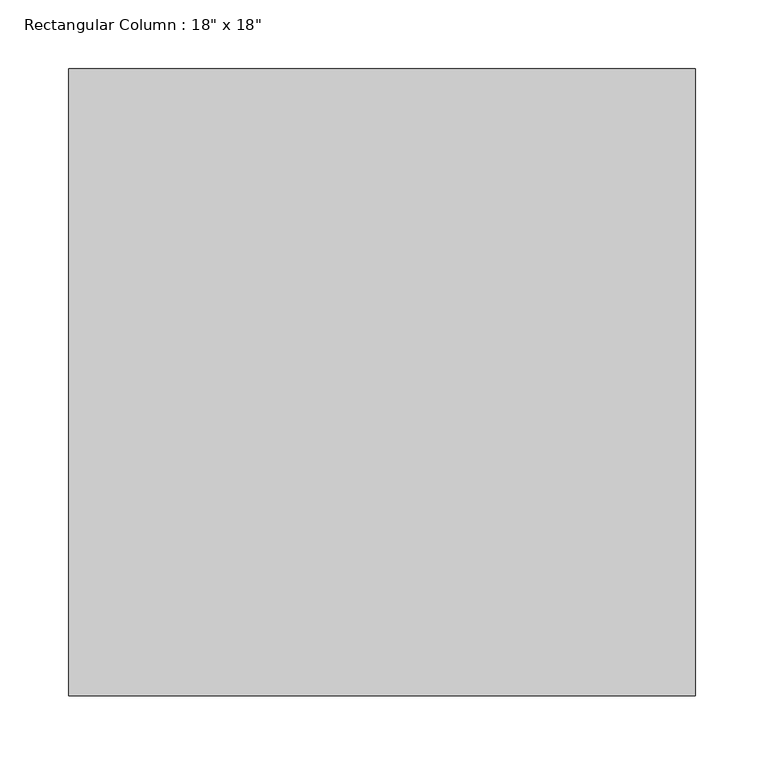
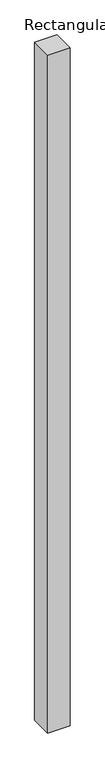
"""IFC4 building model written with IfcOpenShell, lengths in millimetres: column geometry."""

from ifc_helpers import new_model, si_unit, frame, origin, place, context, project, spatial, polyline, outline, extrude, source, transform, mapped, element, save


def column_5762f69e(model_context):
    return source(origin(), model_context, "Body", "SweptSolid", [
        extrude(outline(polyline([(228.6, 228.6), (228.6, -228.6), (-228.6, -228.6), (-228.6, 228.6), (228.6, 228.6)])), frame((0.0, 0.0, 3657.6), z_axis=(0.0, 0.0, 1.0), x_axis=(1.0, 0.0, 0.0)), (0.0, 0.0, 1.0), 14630.4),
    ])


if __name__ == "__main__":
    model = new_model("IFC4")
    model_context = context("Model", 3, world=origin())
    ifc_project = project(units=[si_unit("LENGTHUNIT", "METRE", prefix="MILLI")], contexts=[model_context])
    site = spatial("IfcSite", under=ifc_project)
    building = spatial("IfcBuilding", under=site)
    placement = place(None, origin())
    column_shape = column_5762f69e(model_context)
    element("IfcColumn", 1, ObjectType="Rectangular Column : 18\" x 18\"", at=placement, inside=building, context=model_context, shape_type="MappedRepresentation", body=[
        mapped(column_shape, transform((0.0, 0.0, 0.0), x_axis=(1.0, 0.0, 0.0), y_axis=(0.0, 1.0, 0.0), z_axis=(0.0, 0.0, 1.0))),
    ])
    save(model, "model.ifc")

# Revit data of these elements
# Type "Rectangular Column : 18\" x 18\""
#   Assembly Code = "B1010200"
#   Depth = 1' - 6"
#   Offset Base = 0' - 0"
#   Offset Top = 0' - 0"
#   Width = 1' - 6"
#   Material = none
